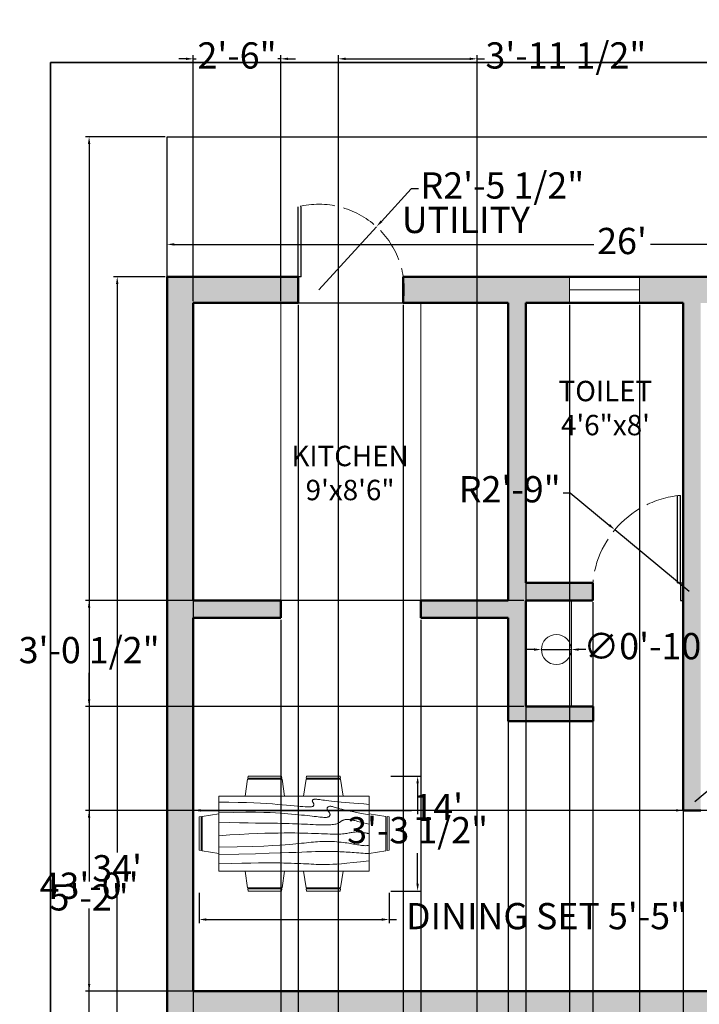
# Model space of a CAD drawing. Units: inches. Extents: x 24899 to 30135, y 37074 to 37745.
# Tile 2 of 3: x 24899 to 25132, y 37333 to 37671. Entities that reach past the tile are written whole.
import ezdxf

# ---------------------------------------------------------------- set-up
doc = ezdxf.new("R2010")
doc.units = ezdxf.units.IN
doc.linetypes.add('ACAD_ISO02W100', pattern=[15, 12, -3])
for name, color, linetype, lineweight in [('A-ANNO-DIMS', 2, 'Continuous', 18), ('A-ANNO-TTLB', 7, 'Continuous', 35), ('A-AREA-IDEN', 7, 'Continuous', 25), ('A-DOOR', 4, 'Continuous', 25), ('A-DOOR-SWNG', 4, 'ACAD_ISO02W100', 13), ('A-FLOR-FIXT', 9, 'Continuous', 18), ('A-FURN', 8, 'Continuous', 18), ('A-GLAZ', 4, 'Continuous', 18), ('A-WALL', 7, 'Continuous', 50), ('C-PROP', 3, 'Continuous', 25)]:
    doc.layers.add(name, color=color, linetype=linetype, lineweight=lineweight)
doc.layers.add('A-WALL-PATT', color=18, linetype='Continuous', lineweight=13, true_color=0x000000)
doc.styles.get("Standard").update_dxf_attribs({"font": 'arial.ttf'})
doc.dimstyles.new('ISO-25', dxfattribs={"dimtxt": 9, "dimasz": 2.5, "dimexe": 1.25, "dimexo": 0.625, "dimgap": 2, "dimtad": 0, "dimtih": 1, "dimtoh": 1, "dimdec": 1, "dimlunit": 4, "dimtxsty": 'Standard', "dimcen": 2.5, "dimadec": 0, "dimazin": 0, "dimtfac": 0.5, "dimtdec": 1, "dimtmove": 0, "dimatfit": 3, "dimfxl": 1, "dimarcsym": 0})

# ---------------------------------------------------------------- blocks, each defined once
blk = doc.blocks.new('*D1')
at = {"layer": 'A-ANNO-DIMS', "color": 0, "lineweight": -2, "transparency": 16777216}
for p, q in [((24949.48, 37583.06), (24949.48, 37594.75)), ((25261.48, 37583.06), (25261.48, 37594.75)), ((24951.98, 37593.5), (25095.76, 37593.5)), ((25258.98, 37593.5), (25115.19, 37593.5))]:
    blk.add_line(p, q, dxfattribs=at)
at = {"layer": 'A-ANNO-DIMS', "color": 0, "transparency": 16777216}
for points in [[(24951.98, 37593.92), (24951.98, 37593.09), (24949.48, 37593.5)], [(25258.98, 37593.92), (25258.98, 37593.09), (25261.48, 37593.5)]]:
    blk.add_solid(points, dxfattribs=at)
at = {"layer": 'Defpoints', "color": 0, "transparency": 16777216}
for p in [(25261.48, 37593.5), (24949.48, 37582.43), (25261.48, 37582.43)]:
    blk.add_point(p, dxfattribs=at)
at = {"layer": 'A-ANNO-DIMS', "color": 0, "transparency": 16777216, "insert": (25105.48, 37593.5), "char_height": 9, "attachment_point": 5}
blk.add_mtext("26'", dxfattribs=at)
blk = doc.blocks.new('*D2')
at = {"layer": 'A-ANNO-DIMS', "color": 0, "lineweight": -2, "transparency": 16777216}
for p, q in [((24948.85, 37582.43), (24931.16, 37582.43)), ((24932.41, 37579.93), (24932.41, 37385.03)), ((24932.41, 37176.93), (24932.41, 37371.83)), ((24948.85, 37174.43), (24931.16, 37174.43))]:
    blk.add_line(p, q, dxfattribs=at)
at = {"layer": 'A-ANNO-DIMS', "color": 0, "transparency": 16777216}
for points in [[(24932, 37579.93), (24932.83, 37579.93), (24932.41, 37582.43)], [(24932, 37176.93), (24932.83, 37176.93), (24932.41, 37174.43)]]:
    blk.add_solid(points, dxfattribs=at)
at = {"layer": 'Defpoints', "color": 0, "transparency": 16777216}
for p in [(24949.48, 37582.43), (24932.41, 37174.43), (24949.48, 37174.43)]:
    blk.add_point(p, dxfattribs=at)
at = {"layer": 'A-ANNO-DIMS', "color": 0, "transparency": 16777216, "insert": (24932.41, 37378.43), "char_height": 9, "attachment_point": 5}
blk.add_mtext("34'", dxfattribs=at)
blk = doc.blocks.new('Dining Set - 36 x 72 in.')
for p, q in [((-22.2343, 26.00059), (-23.4847, 17.99762)), ((-22.2304, 26), (-5.7608, 26)), ((-22, 27.5), (-22.1562, 26.50042)), ((-5.8416, 26.5), (-22.1534, 26.5)), ((-22, 27.5), (-6, 27.5)), ((-5.8437, 26.49966), (-6, 27.5)), ((-4.5152, 17.99762), (-5.7655, 25.99926)), ((5.7657, 26.00059), (4.5153, 17.99762)), ((5.7696, 26), (22.2392, 26)), ((6, 27.5), (5.8438, 26.50042)), ((22.1584, 26.5), (5.8466, 26.5)), ((6, 27.5), (22, 27.5)), ((22.1563, 26.49966), (22, 27.5)), ((23.4848, 17.99762), (22.2345, 25.99926)), ((36, 18), (-36, 18)), ((-36, 18), (-36, -18)), ((36, -18), (36, 18)), ((-44.0006, 8.23428), (-35.9976, 9.48474)), ((44.0006, 8.23428), (35.9976, 9.48474)), ((-45.5, 8), (-44.5004, 8.15617)), ((-45.5, 8), (-45.5, -8)), ((-44.5, -8.15843), (-44.5, 8.15338)), ((-44, 8.23041), (-44, -8.23915)), ((44, 8.23041), (44, -8.23915)), ((44.5, -8.15843), (44.5, 8.15338)), ((45.5, 8), (44.5005, 8.15617)), ((45.5, 8), (45.5, -8)), ((-44.4997, -8.15631), (-45.5, -8)), ((-35.9976, -9.48476), (-43.9993, -8.2345)), ((35.9976, -9.48476), (43.9993, -8.2345)), ((44.4997, -8.15631), (45.5, -8)), ((-36, -18), (36, -18)), ((-22.2343, -26.0006), (-23.4847, -17.99762)), ((-4.5152, -17.99762), (-5.7655, -25.99928)), ((5.7657, -26.0006), (4.5153, -17.99762)), ((23.4848, -17.99762), (22.2345, -25.99928)), ((-22.2304, -26), (-5.7608, -26)), ((-22, -27.5), (-22.1562, -26.50044)), ((-5.8416, -26.5), (-22.1534, -26.5)), ((-22, -27.5), (-6, -27.5)), ((-5.8437, -26.49967), (-6, -27.5)), ((5.7696, -26), (22.2392, -26)), ((6, -27.5), (5.8438, -26.50044)), ((22.1584, -26.5), (5.8466, -26.5)), ((6, -27.5), (22, -27.5)), ((22.1563, -26.49967), (22, -27.5))]:
    blk.add_line(p, q)
for points in [[(-36, 15), (-31.1772, 14.97754), (-26.8079, 14.91406), (-22.8538, 14.81543), (-19.276, 14.6875), (-16.0362, 14.53613), (-13.0957, 14.36718), (-10.4159, 14.18652), (-7.9583, 14), (-5.6904, 13.81315), (-3.6035, 13.63021), (-1.6954, 13.45508), (0.0365, 13.29166), (1.5945, 13.14388), (2.9811, 13.01562), (4.1988, 12.9108), (5.25, 12.83333), (6.1393, 12.78613), (6.8802, 12.76823), (7.4883, 12.77767), (7.9792, 12.8125), (8.3685, 12.87077), (8.6719, 12.95052), (8.9049, 13.0498), (9.0833, 13.16666), (9.2205, 13.29899), (9.3216, 13.44401), (9.3895, 13.59879), (9.4271, 13.76041), (9.4373, 13.92594), (9.4232, 14.09245), (9.3875, 14.257), (9.3333, 14.41666), (9.2638, 14.56917), (9.1836, 14.71484), (9.0975, 14.85465), (9.0104, 14.98958), (8.9272, 15.1206), (8.8529, 15.2487), (8.7922, 15.37483), (8.75, 15.5), (8.7305, 15.62467), (8.7344, 15.74739), (8.7617, 15.86621), (8.8125, 15.97916), (8.8867, 16.08431), (8.9844, 16.17968), (9.1055, 16.26334), (9.25, 16.33333), (9.4189, 16.38802), (9.6172, 16.42708), (9.8506, 16.45052), (10.125, 16.45833), (10.4463, 16.45052), (10.8203, 16.42708), (11.2529, 16.38802), (11.75, 16.33333), (12.3184, 16.26318), (12.9694, 16.17838), (13.7151, 16.07991), (14.5677, 15.96875), (15.5395, 15.84586), (16.6426, 15.71224), (17.8893, 15.56884), (19.2917, 15.41666), (20.859, 15.25667), (22.5879, 15.08984), (24.4721, 14.91715), (26.5052, 14.73958), (28.6809, 14.5581), (30.9929, 14.3737), (33.4347, 14.18733), (36, 14)], [(-36, 10), (-28.9766, 10.14274), (-23.1725, 10.20442), (-18.4241, 10.19775), (-14.5677, 10.13541), (-11.4399, 10.03011), (-8.877, 9.89453), (-6.7154, 9.74137), (-4.7917, 9.58333), (-2.9698, 9.43082), (-1.2246, 9.28515), (0.4415, 9.14534), (2.026, 9.01041), (3.5266, 8.87939), (4.9408, 8.7513), (6.266, 8.62516), (7.5, 8.5), (8.6411, 8.37549), (9.6914, 8.2539), (10.6538, 8.13818), (11.5312, 8.03125), (12.3267, 7.93603), (13.043, 7.85547), (13.6831, 7.79248), (14.25, 7.75), (14.7471, 7.7303), (15.1797, 7.73307), (15.5537, 7.75732), (15.875, 7.80208), (16.1494, 7.86637), (16.3828, 7.94922), (16.5811, 8.04964), (16.75, 8.16666), (16.8944, 8.29915), (17.0143, 8.44531), (17.1089, 8.60319), (17.1771, 8.77083), (17.218, 8.94629), (17.2305, 9.1276), (17.2137, 9.31282), (17.1667, 9.5), (17.0895, 9.6875), (16.987, 9.875), (16.8649, 10.0625), (16.7292, 10.25), (16.5856, 10.4375), (16.4401, 10.625), (16.2985, 10.8125), (16.1667, 11), (16.05, 11.18733), (15.9518, 11.3737), (15.8752, 11.5581), (15.8229, 11.73958), (15.798, 11.91715), (15.8034, 12.08984), (15.842, 12.25667), (15.9167, 12.41666), (16.0295, 12.56836), (16.1784, 12.70833), (16.3605, 12.83268), (16.5729, 12.9375), (16.8127, 13.01888), (17.0768, 13.07291), (17.3625, 13.0957), (17.6667, 13.08333), (17.9894, 13.03312), (18.3418, 12.94726), (18.7382, 12.82918), (19.1927, 12.68229), (19.7195, 12.51001), (20.3327, 12.31575), (21.0465, 12.10294), (21.875, 11.875), (22.8357, 11.63354), (23.959, 11.37304), (25.2786, 11.08618), (26.8282, 10.76562), (28.6414, 10.40405), (30.752, 9.99414), (33.1936, 9.52856), (36, 9)], [(-36, 5.5), (-30.7157, 5.3348), (-26.069, 5.20963), (-21.9946, 5.11767), (-18.4271, 5.05208), (-15.3009, 5.00602), (-12.5508, 4.97265), (-10.1112, 4.94515), (-7.9167, 4.91666), (-5.909, 4.88167), (-4.0586, 4.83984), (-2.3429, 4.79215), (-0.7396, 4.73958), (0.7739, 4.6831), (2.22, 4.6237), (3.6213, 4.56233), (5, 4.5), (6.373, 4.43782), (7.7344, 4.3776), (9.0723, 4.32129), (10.375, 4.27083), (11.6309, 4.22819), (12.8281, 4.19531), (13.9551, 4.17415), (15, 4.16666), (15.954, 4.17448), (16.819, 4.19791), (17.6001, 4.23698), (18.3021, 4.29166), (18.9299, 4.36198), (19.4883, 4.44791), (19.9823, 4.54948), (20.4167, 4.66666), (20.7969, 4.79899), (21.1302, 4.94401), (21.4245, 5.09879), (21.6875, 5.26041), (21.9271, 5.42594), (22.1511, 5.59245), (22.3672, 5.757), (22.5834, 5.91666), (22.8065, 6.06868), (23.0404, 6.21093), (23.2879, 6.34147), (23.5521, 6.45833), (23.8358, 6.55957), (24.142, 6.64323), (24.4735, 6.70735), (24.8334, 6.75), (25.2235, 6.76969), (25.642, 6.76692), (26.0858, 6.74267), (26.5521, 6.69791), (27.0379, 6.63362), (27.5404, 6.55078), (28.0565, 6.45036), (28.5834, 6.33333), (29.1242, 6.19987), (29.7071, 6.04687), (30.3661, 5.87044), (31.1354, 5.66666), (32.0493, 5.43164), (33.142, 5.16146), (34.4475, 4.85221), (36, 4.5)], [(-36, -1), (-30.7915, -0.6591), (-26.0195, -0.38216), (-21.6519, -0.16284), (-17.6563, 0.00521), (-14.0005, 0.12833), (-10.6523, 0.21289), (-7.5796, 0.26522), (-4.75, 0.29166), (-2.134, 0.29793), (0.2878, 0.28711), (2.5317, 0.26163), (4.6146, 0.22396), (6.5529, 0.17651), (8.3633, 0.12174), (10.0623, 0.06209), (11.6667, 0), (13.1899, -0.06201), (14.6341, -0.1211), (15.9982, -0.17432), (17.2813, -0.21875), (18.4823, -0.25147), (19.6003, -0.26953), (20.6343, -0.27002), (21.5834, -0.25), (22.4481, -0.20768), (23.2357, -0.14584), (23.9549, -0.06836), (24.6146, 0.02083), (25.2235, 0.11784), (25.7904, 0.21875), (26.3241, 0.31966), (26.8334, 0.41666), (27.3265, 0.50618), (27.8099, 0.58593), (28.2894, 0.65397), (28.7709, 0.70833), (29.2601, 0.74707), (29.763, 0.76823), (30.2855, 0.76985), (30.8334, 0.75), (31.4088, 0.70784), (31.9994, 0.64713), (32.589, 0.57275), (33.1615, 0.48958), (33.7008, 0.4025), (34.1908, 0.3164), (34.6153, 0.23616), (34.9584, 0.16666), (35.2099, 0.11165), (35.3848, 0.07031), (35.504, 0.04069), (35.5886, 0.02083), (35.6594, 0.00879), (35.7377, 0.0026), (35.8442, 0.00032), (36, 0)], [(-36, -6.5), (-27.1843, -6.31267), (-20.084, -6.1263), (-14.469, -5.9419), (-10.1094, -5.76042), (-6.7752, -5.58285), (-4.2363, -5.41016), (-2.2629, -5.24333), (-0.625, -5.08334), (0.8708, -4.93099), (2.2715, -4.78646), (3.5872, -4.64974), (4.8281, -4.52084), (6.0046, -4.39974), (7.127, -4.28646), (8.2053, -4.18099), (9.25, -4.08334), (10.2705, -3.99382), (11.2734, -3.91407), (12.2647, -3.84603), (13.25, -3.79167), (14.2354, -3.75293), (15.2266, -3.73177), (16.2295, -3.73015), (17.25, -3.75), (18.2912, -3.79248), (19.3451, -3.85547), (20.4009, -3.93604), (21.4479, -4.03125), (22.4754, -4.13819), (23.4727, -4.25391), (24.4289, -4.37549), (25.3334, -4.5), (26.1785, -4.62492), (26.9694, -4.74935), (27.7145, -4.87281), (28.4219, -4.99479), (29.1, -5.11483), (29.7572, -5.23242), (30.4016, -5.34709), (31.0417, -5.45834), (31.6837, -5.56437), (32.3262, -5.65821), (32.9658, -5.73153), (33.599, -5.77604), (34.2224, -5.78345), (34.8327, -5.74545), (35.4264, -5.65373), (36, -5.5)], [(-36, -10), (-26.4022, -9.81299), (-18.4675, -9.62891), (-11.9839, -9.45069), (-6.7396, -9.28125), (-2.5226, -9.12354), (0.8789, -8.98047), (3.6769, -8.85498), (6.0833, -8.75), (8.2767, -8.66765), (10.3021, -8.60677), (12.1712, -8.56543), (13.8958, -8.54167), (15.4876, -8.53353), (16.9583, -8.53907), (18.3197, -8.55632), (19.5834, -8.58334), (20.7616, -8.61841), (21.8685, -8.66081), (22.9188, -8.71004), (23.9271, -8.76563), (24.9081, -8.82707), (25.8763, -8.89388), (26.8465, -8.96558), (27.8334, -9.04167), (28.8474, -9.12118), (29.8828, -9.20117), (30.93, -9.27824), (31.9792, -9.34896), (33.0205, -9.40991), (34.0443, -9.45768), (35.0407, -9.48885), (36, -9.5)], [(-36, -14.5), (-30.0881, -14.33513), (-25.0332, -14.21224), (-20.7312, -14.12647), (-17.0781, -14.07292), (-13.97, -14.04671), (-11.3027, -14.04297), (-8.9724, -14.05681), (-6.875, -14.08334), (-4.9224, -14.11833), (-3.0905, -14.16016), (-1.3709, -14.20785), (0.2448, -14.26042), (1.7647, -14.3169), (3.1973, -14.3763), (4.5507, -14.43767), (5.8333, -14.5), (7.0554, -14.5621), (8.235, -14.62175), (9.3922, -14.67652), (10.5469, -14.72396), (11.7192, -14.76164), (12.929, -14.78711), (14.1965, -14.79794), (15.5417, -14.79167), (16.9933, -14.76424), (18.6152, -14.70508), (20.4804, -14.60197), (22.6615, -14.44271), (25.2312, -14.21509), (28.2624, -13.9069), (31.8277, -13.50594), (36, -13)]]:
    blk.add_lwpolyline(points)
blk = doc.blocks.new('*D4')
at = {"layer": 'A-ANNO-DIMS', "color": 0, "lineweight": -2, "transparency": 16777216}
for p, q in [((24958.48, 37400.06), (24958.48, 37400.68)), ((24960.98, 37399.43), (25033.26, 37399.43)), ((25123.98, 37399.43), (25051.69, 37399.43)), ((25126.48, 37400.06), (25126.48, 37400.68))]:
    blk.add_line(p, q, dxfattribs=at)
at = {"layer": 'A-ANNO-DIMS', "color": 0, "transparency": 16777216}
for points in [[(24960.98, 37399.85), (24960.98, 37399.02), (24958.48, 37399.43)], [(25123.98, 37399.85), (25123.98, 37399.02), (25126.48, 37399.43)]]:
    blk.add_solid(points, dxfattribs=at)
at = {"layer": 'Defpoints', "color": 0, "transparency": 16777216}
for p in [(24958.48, 37399.43), (24958.48, 37399.43), (25126.48, 37399.43)]:
    blk.add_point(p, dxfattribs=at)
at = {"layer": 'A-ANNO-DIMS', "color": 0, "transparency": 16777216, "insert": (25042.48, 37399.43), "char_height": 9, "attachment_point": 5}
blk.add_mtext("14'", dxfattribs=at)
blk = doc.blocks.new('*D13')
at = {"layer": 'A-ANNO-DIMS', "color": 0, "lineweight": -2, "transparency": 16777216}
for p, q in [((24960.47, 37371.15), (24960.47, 37360.75)), ((25025.63, 37371.15), (25025.63, 37360.75)), ((24962.97, 37362), (25023.13, 37362)), ((25025.63, 37362), (25028.13, 37362))]:
    blk.add_line(p, q, dxfattribs=at)
at = {"layer": 'A-ANNO-DIMS', "color": 0, "transparency": 16777216}
for points in [[(24962.97, 37362.42), (24962.97, 37361.59), (24960.47, 37362)], [(25023.13, 37362.42), (25023.13, 37361.59), (25025.63, 37362)]]:
    blk.add_solid(points, dxfattribs=at)
at = {"layer": 'Defpoints', "color": 0, "transparency": 16777216}
for p in [(24960.47, 37371.78), (25025.63, 37371.78), (25025.63, 37362)]:
    blk.add_point(p, dxfattribs=at)
at = {"layer": 'A-ANNO-DIMS', "color": 0, "transparency": 16777216, "insert": (25079.59, 37362), "char_height": 9, "attachment_point": 5}
blk.add_mtext('DINING SET 5\'-5"', dxfattribs=at)
blk = doc.blocks.new('*D14')
at = {"layer": 'A-ANNO-DIMS', "color": 0, "lineweight": -2, "transparency": 16777216}
for p, q in [((25026.25, 37411.15), (25036.65, 37411.15)), ((25035.4, 37408.65), (25035.4, 37398.12)), ((25035.4, 37374.28), (25035.4, 37384.81)), ((25026.25, 37371.78), (25036.65, 37371.78))]:
    blk.add_line(p, q, dxfattribs=at)
at = {"layer": 'A-ANNO-DIMS', "color": 0, "transparency": 16777216}
for points in [[(25034.98, 37408.65), (25035.82, 37408.65), (25035.4, 37411.15)], [(25034.98, 37374.28), (25035.82, 37374.28), (25035.4, 37371.78)]]:
    blk.add_solid(points, dxfattribs=at)
at = {"layer": 'Defpoints', "color": 0, "transparency": 16777216}
for p in [(25025.63, 37411.15), (25035.4, 37411.15), (25025.63, 37371.78)]:
    blk.add_point(p, dxfattribs=at)
at = {"layer": 'A-ANNO-DIMS', "color": 0, "transparency": 16777216, "insert": (25035.4, 37391.47), "char_height": 9, "attachment_point": 5}
blk.add_mtext('3\'-3 1/2"', dxfattribs=at)
blk = doc.blocks.new('*D18')
at = {"layer": 'A-ANNO-DIMS', "color": 0, "lineweight": -2, "transparency": 16777216}
for p, q in [((24948.85, 37630.43), (24921.53, 37630.43)), ((24922.78, 37627.93), (24922.78, 37379.03)), ((24922.78, 37116.93), (24922.78, 37365.83)), ((24948.85, 37114.43), (24921.53, 37114.43))]:
    blk.add_line(p, q, dxfattribs=at)
at = {"layer": 'A-ANNO-DIMS', "color": 0, "transparency": 16777216}
for points in [[(24922.36, 37627.93), (24923.19, 37627.93), (24922.78, 37630.43)], [(24922.36, 37116.93), (24923.19, 37116.93), (24922.78, 37114.43)]]:
    blk.add_solid(points, dxfattribs=at)
at = {"layer": 'Defpoints', "color": 0, "transparency": 16777216}
for p in [(24949.48, 37630.43), (24922.78, 37114.43), (24949.48, 37114.43)]:
    blk.add_point(p, dxfattribs=at)
at = {"layer": 'A-ANNO-DIMS', "color": 0, "transparency": 16777216, "insert": (24922.78, 37372.43), "char_height": 9, "attachment_point": 5}
blk.add_mtext('43\'-0"', dxfattribs=at)
blk = doc.blocks.new('*D19')
at = {"layer": 'A-ANNO-DIMS', "color": 0, "lineweight": -2, "transparency": 16777216}
for p, q in [((24958.48, 37572.81), (24958.48, 37086.48)), ((24994.48, 37572.81), (24994.48, 37086.48)), ((24955.98, 37087.73), (24953.48, 37087.73)), ((24958.48, 37087.73), (24962.52, 37087.73)), ((24994.48, 37087.73), (24990.44, 37087.73)), ((24996.98, 37087.73), (24999.48, 37087.73))]:
    blk.add_line(p, q, dxfattribs=at)
at = {"layer": 'A-ANNO-DIMS', "color": 0, "transparency": 16777216}
for points in [[(24955.98, 37088.15), (24955.98, 37087.32), (24958.48, 37087.73)], [(24996.98, 37088.15), (24996.98, 37087.32), (24994.48, 37087.73)]]:
    blk.add_solid(points, dxfattribs=at)
at = {"layer": 'Defpoints', "color": 0, "transparency": 16777216}
for p in [(24958.48, 37573.43), (24994.48, 37573.43), (24994.48, 37087.73)]:
    blk.add_point(p, dxfattribs=at)
at = {"layer": 'A-ANNO-DIMS', "color": 0, "transparency": 16777216, "insert": (24976.48, 37087.73), "char_height": 9, "attachment_point": 5}
blk.add_mtext('3\'-0"', dxfattribs=at)
blk = doc.blocks.new('*D20')
at = {"layer": 'A-ANNO-DIMS', "color": 0, "lineweight": -2, "transparency": 16777216}
for p, q in [((24994.48, 37572.81), (24994.48, 37086.48)), ((25030.48, 37572.81), (25030.48, 37086.48)), ((24991.98, 37087.73), (24989.48, 37087.73)), ((24994.48, 37087.73), (24998.52, 37087.73)), ((25030.48, 37087.73), (25026.44, 37087.73)), ((25032.98, 37087.73), (25035.48, 37087.73))]:
    blk.add_line(p, q, dxfattribs=at)
at = {"layer": 'A-ANNO-DIMS', "color": 0, "transparency": 16777216}
for points in [[(24991.98, 37088.15), (24991.98, 37087.32), (24994.48, 37087.73)], [(25032.98, 37088.15), (25032.98, 37087.32), (25030.48, 37087.73)]]:
    blk.add_solid(points, dxfattribs=at)
at = {"layer": 'Defpoints', "color": 0, "transparency": 16777216}
for p in [(24994.48, 37573.43), (25030.48, 37573.43), (25030.48, 37087.73)]:
    blk.add_point(p, dxfattribs=at)
at = {"layer": 'A-ANNO-DIMS', "color": 0, "transparency": 16777216, "insert": (25012.48, 37087.73), "char_height": 9, "attachment_point": 5}
blk.add_mtext('3\'-0"', dxfattribs=at)
blk = doc.blocks.new('*D21')
at = {"layer": 'A-ANNO-DIMS', "color": 0, "lineweight": -2, "transparency": 16777216}
for p, q in [((25072.48, 37572.81), (25072.48, 37086.48)), ((25087.48, 37572.81), (25087.48, 37086.48)), ((25074.98, 37087.73), (25084.98, 37087.73)), ((25087.48, 37087.73), (25089.98, 37087.73))]:
    blk.add_line(p, q, dxfattribs=at)
at = {"layer": 'A-ANNO-DIMS', "color": 0, "transparency": 16777216}
for points in [[(25074.98, 37088.15), (25074.98, 37087.32), (25072.48, 37087.73)], [(25084.98, 37088.15), (25084.98, 37087.32), (25087.48, 37087.73)]]:
    blk.add_solid(points, dxfattribs=at)
at = {"layer": 'Defpoints', "color": 0, "transparency": 16777216}
for p in [(25072.48, 37573.43), (25087.48, 37573.43), (25087.48, 37087.73)]:
    blk.add_point(p, dxfattribs=at)
at = {"layer": 'A-ANNO-DIMS', "color": 0, "transparency": 16777216, "insert": (25103.52, 37087.73), "char_height": 9, "attachment_point": 5}
blk.add_mtext('1\'-3"', dxfattribs=at)
blk = doc.blocks.new('*D22')
at = {"layer": 'A-ANNO-DIMS', "color": 0, "lineweight": -2, "transparency": 16777216}
for p, q in [((25087.48, 37572.81), (25087.48, 37086.48)), ((25111.48, 37572.81), (25111.48, 37086.48)), ((25089.98, 37087.73), (25108.98, 37087.73)), ((25111.48, 37087.73), (25113.98, 37087.73))]:
    blk.add_line(p, q, dxfattribs=at)
at = {"layer": 'A-ANNO-DIMS', "color": 0, "transparency": 16777216}
for points in [[(25089.98, 37088.15), (25089.98, 37087.32), (25087.48, 37087.73)], [(25108.98, 37088.15), (25108.98, 37087.32), (25111.48, 37087.73)]]:
    blk.add_solid(points, dxfattribs=at)
at = {"layer": 'Defpoints', "color": 0, "transparency": 16777216}
for p in [(25087.48, 37573.43), (25111.48, 37573.43), (25111.48, 37087.73)]:
    blk.add_point(p, dxfattribs=at)
at = {"layer": 'A-ANNO-DIMS', "color": 0, "transparency": 16777216, "insert": (25128.02, 37087.73), "char_height": 9, "attachment_point": 5}
blk.add_mtext('2\'-0"', dxfattribs=at)
blk = doc.blocks.new('*D25')
at = {"layer": 'A-ANNO-DIMS', "color": 0, "lineweight": -2, "transparency": 16777216}
for p, q in [((24958.48, 37574.06), (24958.48, 37658.38)), ((24988.48, 37574.06), (24988.48, 37658.38)), ((24955.98, 37657.13), (24953.48, 37657.13)), ((24958.48, 37657.13), (24959.44, 37657.13)), ((24988.48, 37657.13), (24987.52, 37657.13)), ((24990.98, 37657.13), (24993.48, 37657.13))]:
    blk.add_line(p, q, dxfattribs=at)
at = {"layer": 'A-ANNO-DIMS', "color": 0, "transparency": 16777216}
for points in [[(24955.98, 37657.55), (24955.98, 37656.72), (24958.48, 37657.13)], [(24990.98, 37657.55), (24990.98, 37656.72), (24988.48, 37657.13)]]:
    blk.add_solid(points, dxfattribs=at)
at = {"layer": 'Defpoints', "color": 0, "transparency": 16777216}
for p in [(24958.48, 37657.13), (24958.48, 37573.43), (24988.48, 37573.43)]:
    blk.add_point(p, dxfattribs=at)
at = {"layer": 'A-ANNO-DIMS', "color": 0, "transparency": 16777216, "insert": (24973.48, 37657.13), "char_height": 9, "attachment_point": 5}
blk.add_mtext('2\'-6"', dxfattribs=at)
blk = doc.blocks.new('*D26')
at = {"layer": 'A-ANNO-DIMS', "color": 0, "lineweight": -2, "transparency": 16777216}
for p, q in [((24988.48, 37464.81), (24988.48, 37086.48)), ((25036.48, 37464.81), (25036.48, 37086.48)), ((24990.98, 37087.73), (24998.33, 37087.73)), ((25033.98, 37087.73), (25026.62, 37087.73))]:
    blk.add_line(p, q, dxfattribs=at)
at = {"layer": 'A-ANNO-DIMS', "color": 0, "transparency": 16777216}
for points in [[(24990.98, 37088.15), (24990.98, 37087.32), (24988.48, 37087.73)], [(25033.98, 37088.15), (25033.98, 37087.32), (25036.48, 37087.73)]]:
    blk.add_solid(points, dxfattribs=at)
at = {"layer": 'Defpoints', "color": 0, "transparency": 16777216}
for p in [(24988.48, 37465.43), (25036.48, 37465.43), (25036.48, 37087.73)]:
    blk.add_point(p, dxfattribs=at)
at = {"layer": 'A-ANNO-DIMS', "color": 0, "transparency": 16777216, "insert": (25012.48, 37087.73), "char_height": 9, "attachment_point": 5}
blk.add_mtext('4\'-0"', dxfattribs=at)
blk = doc.blocks.new('*D27')
at = {"layer": 'A-ANNO-DIMS', "color": 0, "lineweight": -2, "transparency": 16777216}
for p, q in [((25095.48, 37470.81), (25095.48, 37086.48)), ((25126.48, 37470.81), (25126.48, 37086.48)), ((25092.98, 37087.73), (25090.48, 37087.73)), ((25095.48, 37087.73), (25096.94, 37087.73)), ((25126.48, 37087.73), (25125.02, 37087.73)), ((25128.98, 37087.73), (25131.48, 37087.73))]:
    blk.add_line(p, q, dxfattribs=at)
at = {"layer": 'A-ANNO-DIMS', "color": 0, "transparency": 16777216}
for points in [[(25092.98, 37088.15), (25092.98, 37087.32), (25095.48, 37087.73)], [(25128.98, 37088.15), (25128.98, 37087.32), (25126.48, 37087.73)]]:
    blk.add_solid(points, dxfattribs=at)
at = {"layer": 'Defpoints', "color": 0, "transparency": 16777216}
for p in [(25095.48, 37471.43), (25126.48, 37471.43), (25126.48, 37087.73)]:
    blk.add_point(p, dxfattribs=at)
at = {"layer": 'A-ANNO-DIMS', "color": 0, "transparency": 16777216, "insert": (25110.98, 37087.73), "char_height": 9, "attachment_point": 5}
blk.add_mtext('2\'-7"', dxfattribs=at)
blk = doc.blocks.new('*D28')
at = {"layer": 'A-ANNO-DIMS', "color": 0, "lineweight": -2, "transparency": 16777216}
for p, q in [((25071.85, 37471.43), (24921.53, 37471.43)), ((24922.78, 37468.93), (24922.78, 37459.88)), ((24922.78, 37437.51), (24922.78, 37446.57)), ((25071.85, 37435.01), (24921.53, 37435.01))]:
    blk.add_line(p, q, dxfattribs=at)
at = {"layer": 'A-ANNO-DIMS', "color": 0, "transparency": 16777216}
for points in [[(24922.36, 37468.93), (24923.19, 37468.93), (24922.78, 37471.43)], [(24922.36, 37437.51), (24923.19, 37437.51), (24922.78, 37435.01)]]:
    blk.add_solid(points, dxfattribs=at)
at = {"layer": 'Defpoints', "color": 0, "transparency": 16777216}
for p in [(24922.78, 37471.43), (25072.48, 37471.43), (25072.48, 37435.01)]:
    blk.add_point(p, dxfattribs=at)
at = {"layer": 'A-ANNO-DIMS', "color": 0, "transparency": 16777216, "insert": (24922.78, 37453.22), "char_height": 9, "attachment_point": 5}
blk.add_mtext('3\'-0 1/2"', dxfattribs=at)
blk = doc.blocks.new('*D32')
at = {"layer": 'A-ANNO-DIMS', "color": 0, "lineweight": -2, "transparency": 16777216}
for p, q in [((25145.27, 37399.43), (24921.53, 37399.43)), ((24922.78, 37396.93), (24922.78, 37375.03)), ((24922.78, 37339.93), (24922.78, 37361.84)), ((25145.27, 37337.43), (24921.53, 37337.43))]:
    blk.add_line(p, q, dxfattribs=at)
at = {"layer": 'A-ANNO-DIMS', "color": 0, "transparency": 16777216}
for points in [[(24922.36, 37396.93), (24923.19, 37396.93), (24922.78, 37399.43)], [(24922.36, 37339.93), (24923.19, 37339.93), (24922.78, 37337.43)]]:
    blk.add_solid(points, dxfattribs=at)
at = {"layer": 'Defpoints', "color": 0, "transparency": 16777216}
for p in [(24922.78, 37399.43), (25145.9, 37399.43), (25145.9, 37337.43)]:
    blk.add_point(p, dxfattribs=at)
at = {"layer": 'A-ANNO-DIMS', "color": 0, "transparency": 16777216, "insert": (24922.78, 37368.43), "char_height": 9, "attachment_point": 5}
blk.add_mtext('5\'-2"', dxfattribs=at)
blk = doc.blocks.new('*D36')
at = {"layer": 'A-ANNO-DIMS', "color": 0, "lineweight": -2, "transparency": 16777216}
for p, q in [((25008.22, 37251.81), (25008.22, 37658.38)), ((25055.79, 37251.81), (25055.79, 37658.38)), ((25010.72, 37657.13), (25053.29, 37657.13)), ((25055.79, 37657.13), (25058.29, 37657.13))]:
    blk.add_line(p, q, dxfattribs=at)
at = {"layer": 'A-ANNO-DIMS', "color": 0, "transparency": 16777216}
for points in [[(25010.72, 37657.55), (25010.72, 37656.72), (25008.22, 37657.13)], [(25053.29, 37657.55), (25053.29, 37656.72), (25055.79, 37657.13)]]:
    blk.add_solid(points, dxfattribs=at)
at = {"layer": 'Defpoints', "color": 0, "transparency": 16777216}
for p in [(25055.79, 37657.13), (25008.22, 37251.19), (25055.79, 37251.19)]:
    blk.add_point(p, dxfattribs=at)
at = {"layer": 'A-ANNO-DIMS', "color": 0, "transparency": 16777216, "insert": (25086.23, 37657.13), "char_height": 9, "attachment_point": 5}
blk.add_mtext('3\'-11 1/2"', dxfattribs=at)
blk = doc.blocks.new('*D45')
at = {"layer": 'A-ANNO-DIMS', "color": 0, "lineweight": -2, "transparency": 16777216}
for p, q in [((25072.48, 37470.81), (25072.48, 37086.48)), ((25066.48, 37464.81), (25066.48, 37086.48)), ((25063.98, 37087.73), (25061.48, 37087.73)), ((25066.48, 37087.73), (25072.48, 37087.73)), ((25074.98, 37087.73), (25077.48, 37087.73))]:
    blk.add_line(p, q, dxfattribs=at)
at = {"layer": 'A-ANNO-DIMS', "color": 0, "transparency": 16777216}
for points in [[(25063.98, 37088.15), (25063.98, 37087.32), (25066.48, 37087.73)], [(25074.98, 37088.15), (25074.98, 37087.32), (25072.48, 37087.73)]]:
    blk.add_solid(points, dxfattribs=at)
at = {"layer": 'Defpoints', "color": 0, "transparency": 16777216}
for p in [(25072.48, 37471.43), (25066.48, 37465.43), (25072.48, 37087.73)]:
    blk.add_point(p, dxfattribs=at)
at = {"layer": 'A-ANNO-DIMS', "color": 0, "transparency": 16777216, "insert": (25091.44, 37087.73), "char_height": 9, "attachment_point": 5}
blk.add_mtext('0\'-6"', dxfattribs=at)
blk = doc.blocks.new('*D47')
at = {"layer": 'A-ANNO-DIMS', "color": 0, "lineweight": -2, "transparency": 16777216}
for p, q in [((25177.99, 37443.16), (25162.07, 37429.52)), ((25180.49, 37443.16), (25177.99, 37443.16)), ((25130.48, 37402.43), (25160.17, 37427.89))]:
    blk.add_line(p, q, dxfattribs=at)
at = {"layer": 'A-ANNO-DIMS', "color": 0, "transparency": 16777216}
blk.add_solid([(25161.8, 37429.83), (25162.34, 37429.2), (25160.17, 37427.89)], dxfattribs=at)
at = {"layer": 'Defpoints', "color": 0, "transparency": 16777216}
for p in [(25160.17, 37427.89), (25130.48, 37402.43)]:
    blk.add_point(p, dxfattribs=at)
at = {"layer": 'A-ANNO-DIMS', "color": 0, "transparency": 16777216, "insert": (25198.76, 37443.16), "char_height": 9, "attachment_point": 5}
blk.add_mtext('R3\'-3"', dxfattribs=at)
blk = doc.blocks.new('*D48')
at = {"layer": 'A-ANNO-DIMS', "color": 0, "lineweight": -2, "transparency": 16777216}
for p, q in [((25085.25, 37508.37), (25087.75, 37508.37)), ((25087.75, 37508.37), (25101.1, 37497.25)), ((25128.48, 37474.43), (25103.02, 37495.65))]:
    blk.add_line(p, q, dxfattribs=at)
at = {"layer": 'A-ANNO-DIMS', "color": 0, "transparency": 16777216}
blk.add_solid([(25101.37, 37497.57), (25100.83, 37496.93), (25103.02, 37495.65)], dxfattribs=at)
at = {"layer": 'Defpoints', "color": 0, "transparency": 16777216}
for p in [(25103.02, 37495.65), (25128.48, 37474.43)]:
    blk.add_point(p, dxfattribs=at)
at = {"layer": 'A-ANNO-DIMS', "color": 0, "transparency": 16777216, "insert": (25066.98, 37508.37), "char_height": 9, "attachment_point": 5}
blk.add_mtext('R2\'-9"', dxfattribs=at)
blk = doc.blocks.new('*D49')
at = {"layer": 'A-ANNO-DIMS', "color": 0, "lineweight": -2, "transparency": 16777216}
for p, q in [((25033.21, 37612.55), (25023, 37601.41)), ((25035.71, 37612.55), (25033.21, 37612.55)), ((25001.48, 37577.93), (25021.31, 37599.57))]:
    blk.add_line(p, q, dxfattribs=at)
at = {"layer": 'A-ANNO-DIMS', "color": 0, "transparency": 16777216}
blk.add_solid([(25022.69, 37601.69), (25023.3, 37601.13), (25021.31, 37599.57)], dxfattribs=at)
at = {"layer": 'Defpoints', "color": 0, "transparency": 16777216}
for p in [(25021.31, 37599.57), (25001.48, 37577.93)]:
    blk.add_point(p, dxfattribs=at)
at = {"layer": 'A-ANNO-DIMS', "color": 0, "transparency": 16777216, "insert": (25064.46, 37612.55), "char_height": 9, "attachment_point": 5}
blk.add_mtext('R2\'-5 1/2"', dxfattribs=at)
blk = doc.blocks.new('*D50')
at = {"layer": 'A-ANNO-DIMS', "color": 0, "lineweight": -2, "transparency": 16777216}
for p, q in [((25075.33, 37454.58), (25072.83, 37454.58)), ((25077.83, 37454.58), (25088.11, 37454.58)), ((25093.11, 37454.58), (25090.61, 37454.58))]:
    blk.add_line(p, q, dxfattribs=at)
at = {"layer": 'A-ANNO-DIMS', "color": 0, "transparency": 16777216}
for points in [[(25075.33, 37454.99), (25075.33, 37454.16), (25077.83, 37454.58)], [(25090.61, 37455), (25090.61, 37454.16), (25088.11, 37454.58)]]:
    blk.add_solid(points, dxfattribs=at)
at = {"layer": 'Defpoints', "color": 0, "transparency": 16777216}
for p in [(25077.83, 37454.58), (25088.11, 37454.58)]:
    blk.add_point(p, dxfattribs=at)
at = {"layer": 'A-ANNO-DIMS', "color": 0, "transparency": 16777216, "insert": (25125.95, 37454.58), "char_height": 9, "attachment_point": 5}
blk.add_mtext('∅0\'-10 1/2"', dxfattribs=at)

msp = doc.modelspace()

# ---------------------------------------------------------------- hatches: boundary and pattern name
at = {"layer": 'A-WALL-PATT'}
h = msp.add_hatch(color=256, dxfattribs=at)
h.dxf.hatch_style = 1
h.paths.add_polyline_path([(25261.48, 37582.43), (25228.48, 37582.43), (25228.48, 37573.43), (25252.48, 37573.43), (25252.48, 37405.43), (25169.48, 37405.43, -0.038405), (25169.48, 37399.43), (25252.48, 37399.43), (25252.48, 37337.43), (25201.48, 37337.43), (24958.48, 37337.43), (24958.48, 37465.43), (24988.48, 37465.43), (24988.48, 37471.43), (24958.48, 37471.43), (24958.48, 37573.43), (24994.48, 37573.43), (24994.48, 37582.43), (24949.48, 37582.43), (24949.48, 37174.43), (25144.48, 37174.43, -0.042779), (25144.48, 37183.43), (24958.48, 37183.43), (24958.48, 37328.43), (25192.48, 37328.43), (25192.48, 37183.43), (25192.48, 37174.43), (25201.48, 37174.43), (25201.48, 37183.43), (25201.48, 37328.43), (25261.48, 37328.43)])
h.paths.add_polyline_path([(25087.48, 37582.43), (25030.48, 37582.43, -0.077125), (25030.48, 37573.43), (25066.48, 37573.43), (25066.48, 37471.43), (25036.48, 37471.43), (25036.48, 37465.43), (25066.48, 37465.43), (25066.48, 37430.04), (25095.6, 37430.04), (25095.6, 37435.01), (25072.48, 37435.01), (25072.48, 37465.43), (25072.48, 37471.43), (25095.48, 37471.43, -0.045361), (25095.48, 37477.43), (25072.48, 37477.43), (25072.48, 37573.43), (25087.48, 37573.43)], flags=0)
h.paths.add_polyline_path([(25156.48, 37582.43), (25111.48, 37582.43), (25111.48, 37573.43), (25126.48, 37573.43), (25126.48, 37477.43), (25126.48, 37471.43), (25126.48, 37399.43), (25132.48, 37399.43), (25132.48, 37405.43), (25132.48, 37471.43), (25132.48, 37573.43), (25156.48, 37573.43)], flags=17)
h = msp.add_hatch(color=256, dxfattribs=at)
h.dxf.hatch_style = 1
h.paths.add_polyline_path([(25072.48, 37471.43), (25095.48, 37471.43, -0.045361), (25095.48, 37477.43), (25072.48, 37477.43), (25072.48, 37573.43), (25087.48, 37573.43), (25087.48, 37582.43), (25030.48, 37582.43, -0.077125), (25030.48, 37573.43), (25066.48, 37573.43), (25066.48, 37471.43), (25036.48, 37471.43), (25036.48, 37465.43), (25066.48, 37465.43), (25066.48, 37430.04), (25095.6, 37430.04), (25095.6, 37435.01), (25072.48, 37435.01), (25072.48, 37465.43)])

# ---------------------------------------------------------------- linework, layer by layer
at = {"layer": 'A-ANNO-TTLB'}
msp.add_lwpolyline([(24909.5, 37655.83), (25346.61, 37655.83), (25346.61, 37086.99), (24909.5, 37086.99)], close=True, dxfattribs=at)
at = {"layer": 'A-DOOR'}
for p, q in [((24994.48, 37582.43), (24994.48, 37606.43)), ((24995.48, 37582.43), (24995.48, 37606.43)), ((24995.48, 37582.43), (24994.48, 37582.43)), ((24994.48, 37573.43), (25030.48, 37573.43)), ((25124.48, 37477.43), (25124.48, 37507.43)), ((25125.48, 37477.43), (25125.48, 37507.43)), ((25124.48, 37477.43), (25126.48, 37477.43)), ((25125.48, 37477.43), (25125.48, 37471.43)), ((25125.48, 37471.43), (25126.48, 37471.43))]:
    msp.add_line(p, q, dxfattribs=at)
at = {"layer": 'A-DOOR-SWNG'}
for centre, radius, start, end in [((25001.48, 37577.93), 29.35, 351.1796, 103.7995), ((25128.48, 37474.43), 33.14, 95.1944, 185.1944)]:
    msp.add_arc(centre, radius, start, end, dxfattribs=at)
at = {"layer": 'A-FLOR-FIXT'}
for p, q in [((24988.48, 37471.43), (24988.48, 37573.43)), ((25036.48, 37471.43), (25036.48, 37573.43)), ((25088.2, 37471.43), (25088.2, 37435.01))]:
    msp.add_line(p, q, dxfattribs=at)
msp.add_circle((25082.97, 37454.58), 5.14, dxfattribs=at)
at = {"layer": 'A-GLAZ'}
for p, q in [((25087.48, 37573.43), (25087.48, 37582.43)), ((25111.48, 37573.43), (25111.48, 37582.43)), ((25087.48, 37577.93), (25111.48, 37577.93))]:
    msp.add_line(p, q, dxfattribs=at)
at = {"layer": 'A-WALL'}
for p, q in [((24949.48, 37582.43), (24994.48, 37582.43)), ((24949.48, 37582.43), (24949.48, 37174.43)), ((24994.48, 37573.43), (24994.48, 37582.43)), ((25030.48, 37573.43), (25030.48, 37582.43)), ((25030.48, 37582.43), (25261.48, 37582.43)), ((24958.48, 37573.43), (24994.48, 37573.43)), ((24958.48, 37573.43), (24958.48, 37471.43)), ((25030.48, 37573.43), (25066.48, 37573.43)), ((25066.48, 37573.43), (25066.48, 37471.43)), ((25072.48, 37573.43), (25072.48, 37477.43)), ((25072.48, 37573.43), (25126.48, 37573.43)), ((25126.48, 37573.43), (25126.48, 37477.43)), ((25072.48, 37477.43), (25095.48, 37477.43)), ((25095.48, 37477.43), (25095.48, 37471.43)), ((25126.48, 37477.43), (25126.48, 37471.43)), ((24958.48, 37471.43), (24988.48, 37471.43)), ((24988.48, 37465.43), (24988.48, 37471.43)), ((25036.48, 37465.43), (25036.48, 37471.43)), ((25036.48, 37471.43), (25066.48, 37471.43)), ((25072.48, 37471.43), (25095.48, 37471.43)), ((25072.48, 37471.43), (25072.48, 37465.43)), ((25126.48, 37471.43), (25126.48, 37399.43)), ((24958.48, 37465.43), (24988.48, 37465.43)), ((24958.48, 37465.43), (24958.48, 37337.43)), ((25036.48, 37465.43), (25066.48, 37465.43)), ((25066.48, 37465.43), (25066.48, 37430.04)), ((25072.48, 37465.43), (25072.48, 37435.01)), ((25072.48, 37435.01), (25095.48, 37435.01)), ((25095.6, 37430.04), (25095.6, 37435.01)), ((25066.48, 37430.04), (25095.6, 37430.04)), ((25132.48, 37399.43), (25126.48, 37399.43)), ((24958.48, 37337.43), (25201.48, 37337.43))]:
    msp.add_line(p, q, dxfattribs=at)
at = {"layer": 'C-PROP'}
for p, q in [((24949.48, 37582.43), (24949.48, 37630.43)), ((24949.48, 37630.43), (25321.48, 37630.43))]:
    msp.add_line(p, q, dxfattribs=at)

# ---------------------------------------------------------------- block references
at = {"layer": 'A-FURN', "xscale": 0.7159626555889503, "yscale": 0.7159626555889503, "zscale": 0.7159626555889503}
msp.add_blockref('Dining Set - 36 x 72 in.', (24993.05, 37391.47), dxfattribs=at)

# ---------------------------------------------------------------- texts
at = {"layer": 'A-AREA-IDEN', "attachment_point": 1}
for s, width, insert, char_height in [('\\pxqc;UTILITY', 49.0933, (25027.39, 37606.39), 9), ('\\pxqc;{\\fArial|b1|i0|c0|p34;TOILET\\P4\'6"x8\'}', 46.1055, (25076.74, 37546.72), 7), ('\\pxqc;{\\fArial|b1|i0|c0|p34;KITCHEN\\P9\'x8\'6"}', 40.0206, (24992.24, 37524.45), 7)]:
    msp.add_mtext_dynamic_manual_height_columns(s, width=width, gutter_width=12.5, heights=[0], dxfattribs=dict(at, insert=insert, char_height=char_height))

# ---------------------------------------------------------------- dimensions: what is measured, and where the dimension line sits
at = {"layer": 'A-ANNO-DIMS'}
for base, p1, p2, override, picture, middle in [((25055.79, 37657.13), (25008.22, 37251.19), (25055.79, 37251.19), {"dimdec": 1, "dimlfac": 1, "dimrnd": 0, "dimzin": 1, "dimdsep": 46, "dimlunit": 4, "dimfrac": 2}, '*D36', (25086.23, 37657.13)), ((24958.48, 37657.13), (24988.48, 37573.43), (24958.48, 37573.43), {"dimdec": 1, "dimlfac": 1, "dimrnd": 0, "dimzin": 1, "dimdsep": 46, "dimlunit": 4, "dimfrac": 2}, '*D25', (24973.48, 37657.13)), ((25261.48, 37593.5), (24949.48, 37582.43), (25261.48, 37582.43), {"dimclrd": 0, "dimclre": 0, "dimclrt": 0}, '*D1', (25105.48, 37593.5)), ((24994.48, 37087.73), (24958.48, 37573.43), (24994.48, 37573.43), {"dimdec": 1, "dimlfac": 1, "dimrnd": 0, "dimzin": 1, "dimdsep": 46, "dimlunit": 4, "dimfrac": 2}, '*D19', (24976.48, 37087.73)), ((25030.48, 37087.73), (24994.48, 37573.43), (25030.48, 37573.43), {"dimdec": 1, "dimlfac": 1, "dimrnd": 0, "dimzin": 1, "dimdsep": 46, "dimlunit": 4, "dimfrac": 2}, '*D20', (25012.48, 37087.73)), ((25087.48, 37087.73), (25072.48, 37573.43), (25087.48, 37573.43), {"dimdec": 1, "dimlfac": 1, "dimrnd": 0, "dimzin": 1, "dimdsep": 46, "dimlunit": 4, "dimfrac": 2}, '*D21', (25103.52, 37087.73)), ((25111.48, 37087.73), (25087.48, 37573.43), (25111.48, 37573.43), {"dimdec": 1, "dimlfac": 1, "dimrnd": 0, "dimzin": 1, "dimdsep": 46, "dimlunit": 4, "dimfrac": 2}, '*D22', (25128.02, 37087.73)), ((25072.48, 37087.73), (25066.48, 37465.43), (25072.48, 37471.43), {"dimdec": 1, "dimlfac": 1, "dimrnd": 0, "dimzin": 1, "dimdsep": 46, "dimlunit": 4, "dimfrac": 2}, '*D45', (25091.44, 37087.73)), ((25126.48, 37087.73), (25095.48, 37471.43), (25126.48, 37471.43), {"dimdec": 1, "dimlfac": 1, "dimrnd": 0, "dimzin": 1, "dimdsep": 46, "dimlunit": 4, "dimfrac": 2}, '*D27', (25110.98, 37087.73)), ((25036.48, 37087.73), (24988.48, 37465.43), (25036.48, 37465.43), {"dimdec": 1, "dimlfac": 1, "dimrnd": 0, "dimzin": 1, "dimdsep": 46, "dimlunit": 4, "dimfrac": 2}, '*D26', (25012.48, 37087.73)), ((24958.48, 37399.43), (25126.48, 37399.43), (24958.48, 37399.43), {"dimclrd": 0, "dimclre": 0, "dimclrt": 0}, '*D4', (25042.48, 37399.43))]:
    dim = msp.add_linear_dim(base=base, p1=p1, p2=p2, dimstyle='ISO-25', override=override, dxfattribs=at)
    dim.commit()
    dim.dimension.update_dxf_attribs({"geometry": picture, "text_midpoint": middle})
for base, p1, p2, override, picture, middle in [((24922.78, 37114.43), (24949.48, 37630.43), (24949.48, 37114.43), {"dimdec": 1, "dimlfac": 1, "dimrnd": 0, "dimzin": 1, "dimdsep": 46, "dimlunit": 4, "dimfrac": 2}, '*D18', (24922.78, 37372.43)), ((24932.41, 37174.43), (24949.48, 37582.43), (24949.48, 37174.43), {"dimclrd": 0, "dimclre": 0, "dimclrt": 0}, '*D2', (24932.41, 37378.43)), ((24922.78, 37471.43), (25072.48, 37435.01), (25072.48, 37471.43), {"dimdec": 1, "dimlfac": 1, "dimrnd": 0, "dimzin": 1, "dimdsep": 46, "dimlunit": 4, "dimfrac": 2}, '*D28', (24922.78, 37453.22)), ((25035.4, 37411.15), (25025.63, 37371.78), (25025.63, 37411.15), {"dimdec": 1, "dimlfac": 1, "dimrnd": 0, "dimzin": 1, "dimdsep": 46, "dimlunit": 4, "dimfrac": 2}, '*D14', (25035.4, 37391.47)), ((24922.78, 37399.43), (25145.9, 37337.43), (25145.9, 37399.43), {"dimdec": 1, "dimlfac": 1, "dimrnd": 0, "dimzin": 1, "dimdsep": 46, "dimlunit": 4, "dimfrac": 2}, '*D32', (24922.78, 37368.43))]:
    dim = msp.add_linear_dim(base=base, p1=p1, p2=p2, angle=90, dimstyle='ISO-25', override=override, dxfattribs=at)
    dim.commit()
    dim.dimension.update_dxf_attribs({"geometry": picture, "text_midpoint": middle})
for center, mpoint, picture, middle in [((25001.4767, 37577.9329), (25021.3072, 37599.5662), '*D49', (25064.46, 37612.5462)), ((25128.48, 37474.43), (25103.02, 37495.65), '*D48', (25066.98, 37508.37)), ((25130.48, 37402.43), (25160.17, 37427.89), '*D47', (25198.76, 37443.16))]:
    dim = msp.add_radius_dim(center=center, mpoint=mpoint, dimstyle='ISO-25', override={"dimdec": 1, "dimlfac": 1, "dimrnd": 0, "dimzin": 1, "dimdsep": 46, "dimlunit": 4, "dimfrac": 2}, dxfattribs=at)
    dim.commit()
    dim.dimension.update_dxf_attribs({"geometry": picture, "text_midpoint": middle, "dimtype": 164})
dim = msp.add_diameter_dim_2p(p1=(25077.83, 37454.58), p2=(25088.11, 37454.58), dimstyle='ISO-25', override={"dimdec": 1, "dimlfac": 1, "dimrnd": 0, "dimzin": 1, "dimdsep": 46, "dimlunit": 4, "dimfrac": 2}, dxfattribs=at)
dim.commit()
dim.dimension.update_dxf_attribs({"geometry": '*D50', "text_midpoint": (25093.11, 37454.58), "dimtype": 163})
dim = msp.add_linear_dim(base=(25025.63, 37362), p1=(24960.47, 37371.78), p2=(25025.63, 37371.78), text='DINING SET <>', dimstyle='ISO-25', override={"dimdec": 1, "dimlfac": 1, "dimrnd": 0, "dimzin": 1, "dimdsep": 46, "dimlunit": 4, "dimfrac": 2}, dxfattribs=at)
dim.commit()
dim.dimension.update_dxf_attribs({"geometry": '*D13', "text_midpoint": (25079.59, 37362)})

doc.saveas('drawing.dxf')
